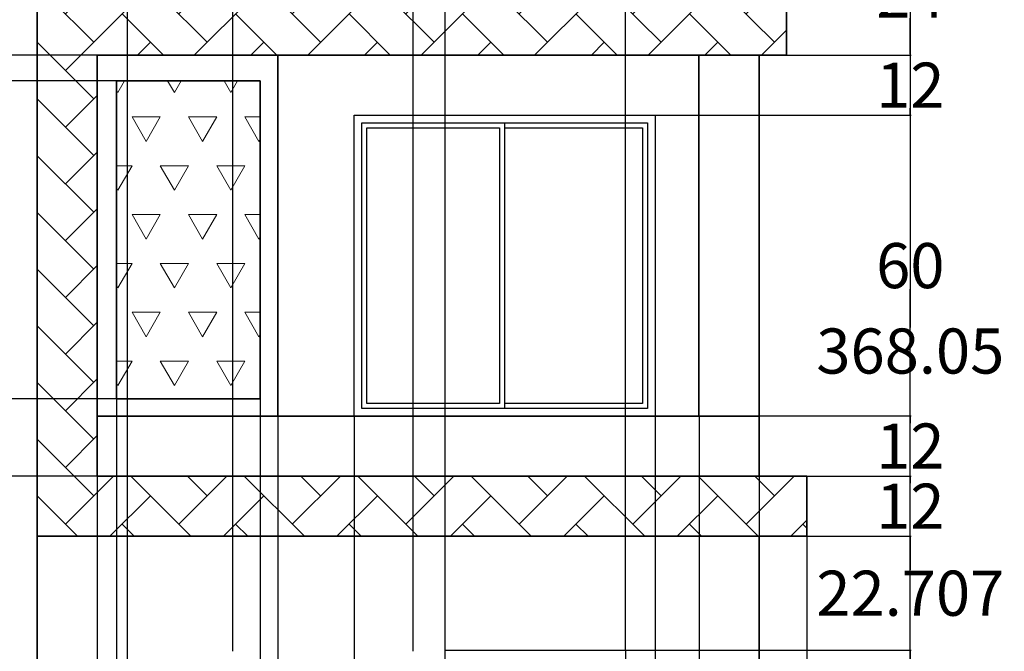
# Model space of a CAD drawing. Units: inches. Extents: x -30 to 323, y -174 to 256.
# Tile 3 of 4: x 127 to 323, y -14 to 112. Entities that reach past the tile are written whole.
import ezdxf

# ---------------------------------------------------------------- set-up
doc = ezdxf.new("R2010")
doc.units = ezdxf.units.IN
doc.header["$MEASUREMENT"] = 0
for name, color, linetype, lineweight in [('A-ANNO-DIMS', 2, 'Continuous', 18), ('A-ELEV', 7, 'Continuous', 35), ('A-ELEV-PATT', 8, 'Continuous', 13), ('A-GLAZ', 3, 'Continuous', 25)]:
    doc.layers.add(name, color=color, linetype=linetype, lineweight=lineweight)
doc.styles.get("Standard").update_dxf_attribs({"font": 'arial.ttf'})
doc.dimstyles.get("Standard").update_dxf_attribs({"dimtxt": 9, "dimasz": 0.18, "dimexe": 0.18, "dimexo": 0.0625, "dimgap": 0.09, "dimtad": 0, "dimtih": 1, "dimtoh": 1, "dimdec": 0, "dimzin": 0, "dimdsep": 46, "dimlunit": 3, "dimtxsty": 'Standard', "dimcen": 0.09, "dimadec": 0, "dimazin": 0, "dimtfac": 1, "dimtdec": 0, "dimtofl": 0, "dimtmove": 0, "dimatfit": 3, "dimfxl": 1, "dimtolj": 1, "dimtzin": 0, "dimarcsym": 0})

# ---------------------------------------------------------------- blocks, each defined once
blk = doc.blocks.new('*U5')
for p, q in [((1.5, 1.5), (1.5, 58.5)), ((1.5, 58.5), (30, 58.5)), ((30, 1.5), (30, 58.5)), ((30, 58.5), (58.5, 58.5)), ((58.5, 58.5), (58.5, 1.5)), ((30, 1.5), (1.5, 1.5)), ((58.5, 1.5), (30, 1.5))]:
    blk.add_line(p, q)
blk.add_lwpolyline([(0, 0), (0, 60), (60, 60), (60, 0)], close=True)
for points in [[(29, 57.5), (29, 2.5), (2.5, 2.5), (2.5, 57.5), (29, 57.5)], [(30, 57.5), (57.5, 57.5), (57.5, 2.5), (30, 2.5)]]:
    blk.add_lwpolyline(points)
blk = doc.blocks.new('*D9')
at = {"layer": 'A-ANNO-DIMS', "color": 0, "lineweight": -2, "transparency": 16777216}
for p, q in [((283.63, 8.84), (283.63, -158.98)), ((22.14, -138.22), (22.14, -158.98)), ((22.32, -158.8), (137.5, -158.8)), ((283.45, -158.8), (168.27, -158.8))]:
    blk.add_line(p, q, dxfattribs=at)
at = {"layer": 'A-ANNO-DIMS', "color": 0, "transparency": 16777216}
for points in [[(22.32, -158.77), (22.32, -158.83), (22.14, -158.8)], [(283.45, -158.77), (283.45, -158.83), (283.63, -158.8)]]:
    blk.add_solid(points, dxfattribs=at)
at = {"layer": 'Defpoints', "color": 0, "transparency": 16777216}
for p in [(283.63, 8.91), (22.14, -138.15), (283.63, -158.8)]:
    blk.add_point(p, dxfattribs=at)
at = {"layer": 'A-ANNO-DIMS', "color": 0, "transparency": 16777216, "insert": (152.88, -158.8), "char_height": 9, "attachment_point": 5}
blk.add_mtext('\\A1;261.5', dxfattribs=at)
blk = doc.blocks.new('*D10')
at = {"layer": 'A-ANNO-DIMS', "color": 0, "lineweight": -2, "transparency": 16777216}
for p, q in [((15.03, 229.9), (304.46, 229.9)), ((304.28, 229.72), (304.28, 50.56)), ((304.28, -137.97), (304.28, 41.18)), ((22.2, -138.15), (304.46, -138.15))]:
    blk.add_line(p, q, dxfattribs=at)
at = {"layer": 'A-ANNO-DIMS', "color": 0, "transparency": 16777216}
for points in [[(304.25, 229.72), (304.31, 229.72), (304.28, 229.9)], [(304.25, -137.97), (304.31, -137.97), (304.28, -138.15)]]:
    blk.add_solid(points, dxfattribs=at)
at = {"layer": 'Defpoints', "color": 0, "transparency": 16777216}
for p in [(14.97, 229.9), (22.14, -138.15), (304.28, -138.15)]:
    blk.add_point(p, dxfattribs=at)
at = {"layer": 'A-ANNO-DIMS', "color": 0, "transparency": 16777216, "insert": (304.28, 45.87), "char_height": 9, "attachment_point": 5}
blk.add_mtext('\\A1;368.05', dxfattribs=at)
blk = doc.blocks.new('*D22')
at = {"layer": 'A-ANNO-DIMS', "color": 0, "lineweight": -2, "transparency": 16777216}
for p, q in [((92.12, -60.62), (92.12, 250.73)), ((92.3, 250.55), (95.9, 250.55)), ((129.96, 250.55), (126.35, 250.55)), ((130.14, -111.03), (130.14, 250.73))]:
    blk.add_line(p, q, dxfattribs=at)
at = {"layer": 'A-ANNO-DIMS', "color": 0, "transparency": 16777216}
for points in [[(92.3, 250.58), (92.3, 250.52), (92.12, 250.55)], [(129.96, 250.58), (129.96, 250.52), (130.14, 250.55)]]:
    blk.add_solid(points, dxfattribs=at)
at = {"layer": 'Defpoints', "color": 0, "transparency": 16777216}
for p in [(130.14, 250.55), (92.12, -60.68), (130.14, -111.09)]:
    blk.add_point(p, dxfattribs=at)
at = {"layer": 'A-ANNO-DIMS', "color": 0, "transparency": 16777216, "insert": (111.13, 250.55), "char_height": 9, "attachment_point": 5}
blk.add_mtext('\\A1;38.02', dxfattribs=at)
blk = doc.blocks.new('*D44')
at = {"layer": 'A-ANNO-DIMS', "color": 0, "lineweight": -2, "transparency": 16777216}
for p, q in [((142.14, 20.84), (142.14, -158.98)), ((130.14, 8.84), (130.14, -158.98)), ((130.32, -158.8), (141.96, -158.8)), ((142.14, -158.8), (142.32, -158.8))]:
    blk.add_line(p, q, dxfattribs=at)
at = {"layer": 'A-ANNO-DIMS', "color": 0, "transparency": 16777216}
for points in [[(130.32, -158.77), (130.32, -158.83), (130.14, -158.8)], [(141.96, -158.77), (141.96, -158.83), (142.14, -158.8)]]:
    blk.add_solid(points, dxfattribs=at)
at = {"layer": 'Defpoints', "color": 0, "transparency": 16777216}
for p in [(142.14, 20.91), (130.14, 8.91), (142.14, -158.8)]:
    blk.add_point(p, dxfattribs=at)
at = {"layer": 'A-ANNO-DIMS', "color": 0, "transparency": 16777216, "insert": (148.38, -158.8), "char_height": 9, "attachment_point": 5}
blk.add_mtext('\\A1;12', dxfattribs=at)
blk = doc.blocks.new('*D45')
at = {"layer": 'A-ANNO-DIMS', "color": 0, "lineweight": -2, "transparency": 16777216}
for p, q in [((145.99, 36.26), (145.99, -158.98)), ((142.14, 20.84), (142.14, -158.98)), ((142.32, -158.8), (145.81, -158.8)), ((145.99, -158.8), (146.17, -158.8))]:
    blk.add_line(p, q, dxfattribs=at)
at = {"layer": 'A-ANNO-DIMS', "color": 0, "transparency": 16777216}
for points in [[(142.32, -158.77), (142.32, -158.83), (142.14, -158.8)], [(145.81, -158.77), (145.81, -158.83), (145.99, -158.8)]]:
    blk.add_solid(points, dxfattribs=at)
at = {"layer": 'Defpoints', "color": 0, "transparency": 16777216}
for p in [(145.99, 36.33), (142.14, 20.91), (145.99, -158.8)]:
    blk.add_point(p, dxfattribs=at)
at = {"layer": 'A-ANNO-DIMS', "color": 0, "transparency": 16777216, "insert": (157.98, -158.8), "char_height": 9, "attachment_point": 5}
blk.add_mtext('\\A1;3.85', dxfattribs=at)
blk = doc.blocks.new('*D46')
at = {"layer": 'A-ANNO-DIMS', "color": 0, "lineweight": -2, "transparency": 16777216}
for p, q in [((145.99, 36.26), (145.99, -158.98)), ((174.62, 36.26), (174.62, -158.98)), ((146.17, -158.8), (174.44, -158.8)), ((174.62, -158.8), (174.8, -158.8))]:
    blk.add_line(p, q, dxfattribs=at)
at = {"layer": 'A-ANNO-DIMS', "color": 0, "transparency": 16777216}
for points in [[(146.17, -158.77), (146.17, -158.83), (145.99, -158.8)], [(174.44, -158.77), (174.44, -158.83), (174.62, -158.8)]]:
    blk.add_solid(points, dxfattribs=at)
at = {"layer": 'Defpoints', "color": 0, "transparency": 16777216}
for p in [(145.99, 36.33), (174.62, 36.33), (174.62, -158.8)]:
    blk.add_point(p, dxfattribs=at)
at = {"layer": 'A-ANNO-DIMS', "color": 0, "transparency": 16777216, "insert": (190.15, -158.8), "char_height": 9, "attachment_point": 5}
blk.add_mtext('\\A1;28.63', dxfattribs=at)
blk = doc.blocks.new('*D47')
at = {"layer": 'A-ANNO-DIMS', "color": 0, "lineweight": -2, "transparency": 16777216}
for p, q in [((174.62, 36.26), (174.62, -158.98)), ((178.14, 32.84), (178.14, -158.98)), ((174.8, -158.8), (177.96, -158.8)), ((178.14, -158.8), (178.32, -158.8))]:
    blk.add_line(p, q, dxfattribs=at)
at = {"layer": 'A-ANNO-DIMS', "color": 0, "transparency": 16777216}
for points in [[(174.8, -158.77), (174.8, -158.83), (174.62, -158.8)], [(177.96, -158.77), (177.96, -158.83), (178.14, -158.8)]]:
    blk.add_solid(points, dxfattribs=at)
at = {"layer": 'Defpoints', "color": 0, "transparency": 16777216}
for p in [(174.62, 36.33), (178.14, 32.91), (178.14, -158.8)]:
    blk.add_point(p, dxfattribs=at)
at = {"layer": 'A-ANNO-DIMS', "color": 0, "transparency": 16777216, "insert": (193.6, -158.8), "char_height": 9, "attachment_point": 5}
blk.add_mtext('\\A1;3.518', dxfattribs=at)
blk = doc.blocks.new('*D48')
at = {"layer": 'A-ANNO-DIMS', "color": 0, "lineweight": -2, "transparency": 16777216}
for p, q in [((178.14, 32.84), (178.14, -158.98)), ((193.38, 32.84), (193.38, -158.98)), ((178.32, -158.8), (193.2, -158.8)), ((193.38, -158.8), (193.56, -158.8))]:
    blk.add_line(p, q, dxfattribs=at)
at = {"layer": 'A-ANNO-DIMS', "color": 0, "transparency": 16777216}
for points in [[(178.32, -158.77), (178.32, -158.83), (178.14, -158.8)], [(193.2, -158.77), (193.2, -158.83), (193.38, -158.8)]]:
    blk.add_solid(points, dxfattribs=at)
at = {"layer": 'Defpoints', "color": 0, "transparency": 16777216}
for p in [(178.14, 32.91), (193.38, 32.91), (193.38, -158.8)]:
    blk.add_point(p, dxfattribs=at)
at = {"layer": 'A-ANNO-DIMS', "color": 0, "transparency": 16777216, "insert": (211.91, -158.8), "char_height": 9, "attachment_point": 5}
blk.add_mtext('\\A1;15.247', dxfattribs=at)
blk = doc.blocks.new('*D49')
at = {"layer": 'A-ANNO-DIMS', "color": 0, "lineweight": -2, "transparency": 16777216}
for p, q in [((193.38, 32.84), (193.38, -158.98)), ((253.38, 32.84), (253.38, -158.98)), ((193.56, -158.8), (216.84, -158.8)), ((253.2, -158.8), (229.93, -158.8))]:
    blk.add_line(p, q, dxfattribs=at)
at = {"layer": 'A-ANNO-DIMS', "color": 0, "transparency": 16777216}
for points in [[(193.56, -158.77), (193.56, -158.83), (193.38, -158.8)], [(253.2, -158.77), (253.2, -158.83), (253.38, -158.8)]]:
    blk.add_solid(points, dxfattribs=at)
at = {"layer": 'Defpoints', "color": 0, "transparency": 16777216}
for p in [(193.38, 32.91), (253.38, 32.91), (253.38, -158.8)]:
    blk.add_point(p, dxfattribs=at)
at = {"layer": 'A-ANNO-DIMS', "color": 0, "transparency": 16777216, "insert": (223.38, -158.8), "char_height": 9, "attachment_point": 5}
blk.add_mtext('\\A1;60', dxfattribs=at)
blk = doc.blocks.new('*D50')
at = {"layer": 'A-ANNO-DIMS', "color": 0, "lineweight": -2, "transparency": 16777216}
for p, q in [((253.38, 32.84), (253.38, -158.98)), ((262.14, 32.84), (262.14, -158.98)), ((253.56, -158.8), (261.96, -158.8)), ((262.14, -158.8), (262.32, -158.8))]:
    blk.add_line(p, q, dxfattribs=at)
at = {"layer": 'A-ANNO-DIMS', "color": 0, "transparency": 16777216}
for points in [[(253.56, -158.77), (253.56, -158.83), (253.38, -158.8)], [(261.96, -158.77), (261.96, -158.83), (262.14, -158.8)]]:
    blk.add_solid(points, dxfattribs=at)
at = {"layer": 'Defpoints', "color": 0, "transparency": 16777216}
for p in [(253.38, 32.91), (262.14, 32.91), (262.14, -158.8)]:
    blk.add_point(p, dxfattribs=at)
at = {"layer": 'A-ANNO-DIMS', "color": 0, "transparency": 16777216, "insert": (277.6, -158.8), "char_height": 9, "attachment_point": 5}
blk.add_mtext('\\A1;8.753', dxfattribs=at)
blk = doc.blocks.new('*D51')
at = {"layer": 'A-ANNO-DIMS', "color": 0, "lineweight": -2, "transparency": 16777216}
for p, q in [((262.14, 32.84), (262.14, -158.98)), ((274.14, 20.84), (274.14, -158.98)), ((262.32, -158.8), (273.96, -158.8)), ((274.14, -158.8), (274.32, -158.8))]:
    blk.add_line(p, q, dxfattribs=at)
at = {"layer": 'A-ANNO-DIMS', "color": 0, "transparency": 16777216}
for points in [[(262.32, -158.77), (262.32, -158.83), (262.14, -158.8)], [(273.96, -158.77), (273.96, -158.83), (274.14, -158.8)]]:
    blk.add_solid(points, dxfattribs=at)
at = {"layer": 'Defpoints', "color": 0, "transparency": 16777216}
for p in [(262.14, 32.91), (274.14, 20.91), (274.14, -158.8)]:
    blk.add_point(p, dxfattribs=at)
at = {"layer": 'A-ANNO-DIMS', "color": 0, "transparency": 16777216, "insert": (280.38, -158.8), "char_height": 9, "attachment_point": 5}
blk.add_mtext('\\A1;12', dxfattribs=at)
blk = doc.blocks.new('*D52')
at = {"layer": 'A-ANNO-DIMS', "color": 0, "lineweight": -2, "transparency": 16777216}
for p, q in [((148.14, -47.95), (148.14, 250.73)), ((148.32, 250.55), (168.97, 250.55)), ((169.15, -13.98), (169.15, 250.73)), ((169.15, 250.55), (169.33, 250.55))]:
    blk.add_line(p, q, dxfattribs=at)
at = {"layer": 'A-ANNO-DIMS', "color": 0, "transparency": 16777216}
for points in [[(148.32, 250.58), (148.32, 250.52), (148.14, 250.55)], [(168.97, 250.58), (168.97, 250.52), (169.15, 250.55)]]:
    blk.add_solid(points, dxfattribs=at)
at = {"layer": 'Defpoints', "color": 0, "transparency": 16777216}
for p in [(169.15, 250.55), (169.15, -14.04), (148.14, -48.01)]:
    blk.add_point(p, dxfattribs=at)
at = {"layer": 'A-ANNO-DIMS', "color": 0, "transparency": 16777216, "insert": (188.16, 250.55), "char_height": 9, "attachment_point": 5}
blk.add_mtext('\\A1;21.014', dxfattribs=at)
blk = doc.blocks.new('*D53')
at = {"layer": 'A-ANNO-DIMS', "color": 0, "lineweight": -2, "transparency": 16777216}
for p, q in [((169.15, -13.98), (169.15, 250.73)), ((169.33, 250.55), (180.62, 250.55)), ((204.97, 250.55), (193.68, 250.55)), ((205.15, -13.98), (205.15, 250.73))]:
    blk.add_line(p, q, dxfattribs=at)
at = {"layer": 'A-ANNO-DIMS', "color": 0, "transparency": 16777216}
for points in [[(169.33, 250.58), (169.33, 250.52), (169.15, 250.55)], [(204.97, 250.58), (204.97, 250.52), (205.15, 250.55)]]:
    blk.add_solid(points, dxfattribs=at)
at = {"layer": 'Defpoints', "color": 0, "transparency": 16777216}
for p in [(205.15, 250.55), (169.15, -14.04), (205.15, -14.04)]:
    blk.add_point(p, dxfattribs=at)
at = {"layer": 'A-ANNO-DIMS', "color": 0, "transparency": 16777216, "insert": (187.15, 250.55), "char_height": 9, "attachment_point": 5}
blk.add_mtext('\\A1;36', dxfattribs=at)
blk = doc.blocks.new('*D54')
at = {"layer": 'A-ANNO-DIMS', "color": 0, "lineweight": -2, "transparency": 16777216}
for p, q in [((205.15, -13.98), (205.15, 250.73)), ((205.33, 250.55), (211.31, 250.55)), ((211.49, -13.74), (211.49, 250.73)), ((211.49, 250.55), (211.67, 250.55))]:
    blk.add_line(p, q, dxfattribs=at)
at = {"layer": 'A-ANNO-DIMS', "color": 0, "transparency": 16777216}
for points in [[(205.33, 250.58), (205.33, 250.52), (205.15, 250.55)], [(211.31, 250.58), (211.31, 250.52), (211.49, 250.55)]]:
    blk.add_solid(points, dxfattribs=at)
at = {"layer": 'Defpoints', "color": 0, "transparency": 16777216}
for p in [(211.49, 250.55), (205.15, -14.04), (211.49, -13.8)]:
    blk.add_point(p, dxfattribs=at)
at = {"layer": 'A-ANNO-DIMS', "color": 0, "transparency": 16777216, "insert": (226.98, 250.55), "char_height": 9, "attachment_point": 5}
blk.add_mtext('\\A1;6.338', dxfattribs=at)
blk = doc.blocks.new('*D55')
at = {"layer": 'A-ANNO-DIMS', "color": 0, "lineweight": -2, "transparency": 16777216}
for p, q in [((211.49, -13.74), (211.49, 250.73)), ((211.67, 250.55), (222.96, 250.55)), ((247.31, 250.55), (236.02, 250.55)), ((247.49, -13.74), (247.49, 250.73))]:
    blk.add_line(p, q, dxfattribs=at)
at = {"layer": 'A-ANNO-DIMS', "color": 0, "transparency": 16777216}
for points in [[(211.67, 250.58), (211.67, 250.52), (211.49, 250.55)], [(247.31, 250.58), (247.31, 250.52), (247.49, 250.55)]]:
    blk.add_solid(points, dxfattribs=at)
at = {"layer": 'Defpoints', "color": 0, "transparency": 16777216}
for p in [(247.49, 250.55), (211.49, -13.8), (247.49, -13.8)]:
    blk.add_point(p, dxfattribs=at)
at = {"layer": 'A-ANNO-DIMS', "color": 0, "transparency": 16777216, "insert": (229.49, 250.55), "char_height": 9, "attachment_point": 5}
blk.add_mtext('\\A1;36', dxfattribs=at)
blk = doc.blocks.new('*D60')
at = {"layer": 'A-ANNO-DIMS', "color": 0, "lineweight": -2, "transparency": 16777216}
for p, q in [((283.63, 8.84), (283.63, -158.98)), ((274.14, -111.16), (274.14, -158.98)), ((274.32, -158.8), (283.45, -158.8)), ((283.63, -158.8), (283.81, -158.8))]:
    blk.add_line(p, q, dxfattribs=at)
at = {"layer": 'A-ANNO-DIMS', "color": 0, "transparency": 16777216}
for points in [[(274.32, -158.77), (274.32, -158.83), (274.14, -158.8)], [(283.45, -158.77), (283.45, -158.83), (283.63, -158.8)]]:
    blk.add_solid(points, dxfattribs=at)
at = {"layer": 'Defpoints', "color": 0, "transparency": 16777216}
for p in [(283.63, 8.91), (274.14, -111.09), (283.63, -158.8)]:
    blk.add_point(p, dxfattribs=at)
at = {"layer": 'A-ANNO-DIMS', "color": 0, "transparency": 16777216, "insert": (299.09, -158.8), "char_height": 9, "attachment_point": 5}
blk.add_mtext('\\A1;9.497', dxfattribs=at)
blk = doc.blocks.new('*D63')
at = {"layer": 'A-ANNO-DIMS', "color": 0, "lineweight": -2, "transparency": 16777216}
for p, q in [((247.55, -13.8), (304.46, -13.8)), ((304.28, -13.98), (304.28, -26.22)), ((304.28, -47.83), (304.28, -35.59)), ((256.2, -48.01), (304.46, -48.01))]:
    blk.add_line(p, q, dxfattribs=at)
at = {"layer": 'A-ANNO-DIMS', "color": 0, "transparency": 16777216}
for points in [[(304.25, -13.98), (304.31, -13.98), (304.28, -13.8)], [(304.25, -47.83), (304.31, -47.83), (304.28, -48.01)]]:
    blk.add_solid(points, dxfattribs=at)
at = {"layer": 'Defpoints', "color": 0, "transparency": 16777216}
for p in [(247.49, -13.8), (304.28, -13.8), (256.14, -48.01)]:
    blk.add_point(p, dxfattribs=at)
at = {"layer": 'A-ANNO-DIMS', "color": 0, "transparency": 16777216, "insert": (304.28, -30.9), "char_height": 9, "attachment_point": 5}
blk.add_mtext('\\A1;34.21', dxfattribs=at)
blk = doc.blocks.new('*D64')
at = {"layer": 'A-ANNO-DIMS', "color": 0, "lineweight": -2, "transparency": 16777216}
for p, q in [((283.7, 8.91), (304.46, 8.91)), ((304.28, 8.73), (304.28, 2.24)), ((304.28, -13.62), (304.28, -7.13)), ((247.55, -13.8), (304.46, -13.8))]:
    blk.add_line(p, q, dxfattribs=at)
at = {"layer": 'A-ANNO-DIMS', "color": 0, "transparency": 16777216}
for points in [[(304.25, 8.73), (304.31, 8.73), (304.28, 8.91)], [(304.25, -13.62), (304.31, -13.62), (304.28, -13.8)]]:
    blk.add_solid(points, dxfattribs=at)
at = {"layer": 'Defpoints', "color": 0, "transparency": 16777216}
for p in [(283.63, 8.91), (304.28, 8.91), (247.49, -13.8)]:
    blk.add_point(p, dxfattribs=at)
at = {"layer": 'A-ANNO-DIMS', "color": 0, "transparency": 16777216, "insert": (304.28, -2.45), "char_height": 9, "attachment_point": 5}
blk.add_mtext('\\A1;22.707', dxfattribs=at)
blk = doc.blocks.new('*D65')
at = {"layer": 'A-ANNO-DIMS', "color": 0, "lineweight": -2, "transparency": 16777216}
for p, q in [((283.7, 20.91), (304.46, 20.91)), ((304.28, 20.73), (304.28, 19.51)), ((304.28, 9.09), (304.28, 10.3)), ((283.7, 8.91), (304.46, 8.91))]:
    blk.add_line(p, q, dxfattribs=at)
at = {"layer": 'A-ANNO-DIMS', "color": 0, "transparency": 16777216}
for points in [[(304.25, 20.73), (304.31, 20.73), (304.28, 20.91)], [(304.25, 9.09), (304.31, 9.09), (304.28, 8.91)]]:
    blk.add_solid(points, dxfattribs=at)
at = {"layer": 'Defpoints', "color": 0, "transparency": 16777216}
for p in [(283.63, 20.91), (304.28, 20.91), (283.63, 8.91)]:
    blk.add_point(p, dxfattribs=at)
at = {"layer": 'A-ANNO-DIMS', "color": 0, "transparency": 16777216, "insert": (304.28, 14.91), "char_height": 9, "attachment_point": 5}
blk.add_mtext('\\A1;12', dxfattribs=at)
blk = doc.blocks.new('*D66')
at = {"layer": 'A-ANNO-DIMS', "color": 0, "lineweight": -2, "transparency": 16777216}
for p, q in [((274.2, 32.91), (304.46, 32.91)), ((304.28, 32.73), (304.28, 31.51)), ((304.28, 21.09), (304.28, 22.3)), ((274.2, 20.91), (304.46, 20.91))]:
    blk.add_line(p, q, dxfattribs=at)
at = {"layer": 'A-ANNO-DIMS', "color": 0, "transparency": 16777216}
for points in [[(304.25, 32.73), (304.31, 32.73), (304.28, 32.91)], [(304.25, 21.09), (304.31, 21.09), (304.28, 20.91)]]:
    blk.add_solid(points, dxfattribs=at)
at = {"layer": 'Defpoints', "color": 0, "transparency": 16777216}
for p in [(274.14, 32.91), (304.28, 32.91), (274.14, 20.91)]:
    blk.add_point(p, dxfattribs=at)
at = {"layer": 'A-ANNO-DIMS', "color": 0, "transparency": 16777216, "insert": (304.28, 26.91), "char_height": 9, "attachment_point": 5}
blk.add_mtext('\\A1;12', dxfattribs=at)
blk = doc.blocks.new('*D67')
at = {"layer": 'A-ANNO-DIMS', "color": 0, "lineweight": -2, "transparency": 16777216}
for p, q in [((253.45, 92.91), (304.46, 92.91)), ((304.28, 92.73), (304.28, 67.59)), ((304.28, 33.09), (304.28, 58.22)), ((274.2, 32.91), (304.46, 32.91))]:
    blk.add_line(p, q, dxfattribs=at)
at = {"layer": 'A-ANNO-DIMS', "color": 0, "transparency": 16777216}
for points in [[(304.25, 92.73), (304.31, 92.73), (304.28, 92.91)], [(304.25, 33.09), (304.31, 33.09), (304.28, 32.91)]]:
    blk.add_solid(points, dxfattribs=at)
at = {"layer": 'Defpoints', "color": 0, "transparency": 16777216}
for p in [(253.38, 92.91), (304.28, 92.91), (274.14, 32.91)]:
    blk.add_point(p, dxfattribs=at)
at = {"layer": 'A-ANNO-DIMS', "color": 0, "transparency": 16777216, "insert": (304.28, 62.91), "char_height": 9, "attachment_point": 5}
blk.add_mtext('\\A1;60', dxfattribs=at)
blk = doc.blocks.new('*D68')
at = {"layer": 'A-ANNO-DIMS', "color": 0, "lineweight": -2, "transparency": 16777216}
for p, q in [((274.2, 104.91), (304.46, 104.91)), ((304.28, 104.73), (304.28, 103.51)), ((304.28, 93.09), (304.28, 94.3)), ((253.45, 92.91), (304.46, 92.91))]:
    blk.add_line(p, q, dxfattribs=at)
at = {"layer": 'A-ANNO-DIMS', "color": 0, "transparency": 16777216}
for points in [[(304.25, 104.73), (304.31, 104.73), (304.28, 104.91)], [(304.25, 93.09), (304.31, 93.09), (304.28, 92.91)]]:
    blk.add_solid(points, dxfattribs=at)
at = {"layer": 'Defpoints', "color": 0, "transparency": 16777216}
for p in [(274.14, 104.91), (304.28, 104.91), (253.38, 92.91)]:
    blk.add_point(p, dxfattribs=at)
at = {"layer": 'A-ANNO-DIMS', "color": 0, "transparency": 16777216, "insert": (304.28, 98.91), "char_height": 9, "attachment_point": 5}
blk.add_mtext('\\A1;12', dxfattribs=at)
blk = doc.blocks.new('*D69')
at = {"layer": 'A-ANNO-DIMS', "color": 0, "lineweight": -2, "transparency": 16777216}
for p, q in [((279.63, 128.91), (304.46, 128.91)), ((304.28, 128.73), (304.28, 121.51)), ((304.28, 105.09), (304.28, 112.3)), ((279.63, 104.91), (304.46, 104.91))]:
    blk.add_line(p, q, dxfattribs=at)
at = {"layer": 'A-ANNO-DIMS', "color": 0, "transparency": 16777216}
for points in [[(304.25, 128.73), (304.31, 128.73), (304.28, 128.91)], [(304.25, 105.09), (304.31, 105.09), (304.28, 104.91)]]:
    blk.add_solid(points, dxfattribs=at)
at = {"layer": 'Defpoints', "color": 0, "transparency": 16777216}
for p in [(279.57, 128.91), (304.28, 128.91), (279.57, 104.91)]:
    blk.add_point(p, dxfattribs=at)
at = {"layer": 'A-ANNO-DIMS', "color": 0, "transparency": 16777216, "insert": (304.28, 116.91), "char_height": 9, "attachment_point": 5}
blk.add_mtext('\\A1;24', dxfattribs=at)
blk = doc.blocks.new('*D74')
at = {"layer": 'A-ANNO-DIMS', "color": 0, "lineweight": -2, "transparency": 16777216}
for p, q in [((145.92, 36.33), (-5.86, 36.33)), ((-5.68, 36.15), (-5.68, 33.3)), ((-5.68, 21.09), (-5.68, 23.93)), ((142.07, 20.91), (-5.86, 20.91))]:
    blk.add_line(p, q, dxfattribs=at)
at = {"layer": 'A-ANNO-DIMS', "color": 0, "transparency": 16777216}
for points in [[(-5.71, 36.15), (-5.65, 36.15), (-5.68, 36.33)], [(-5.71, 21.09), (-5.65, 21.09), (-5.68, 20.91)]]:
    blk.add_solid(points, dxfattribs=at)
at = {"layer": 'Defpoints', "color": 0, "transparency": 16777216}
for p in [(-5.68, 36.33), (145.99, 36.33), (142.14, 20.91)]:
    blk.add_point(p, dxfattribs=at)
at = {"layer": 'A-ANNO-DIMS', "color": 0, "transparency": 16777216, "insert": (-5.68, 28.62), "char_height": 9, "attachment_point": 5}
blk.add_mtext('\\A1;15.42', dxfattribs=at)
blk = doc.blocks.new('*D75')
at = {"layer": 'A-ANNO-DIMS', "color": 0, "lineweight": -2, "transparency": 16777216}
for p, q in [((145.92, 99.75), (-5.86, 99.75)), ((-5.68, 99.57), (-5.68, 72.73)), ((-5.68, 36.51), (-5.68, 63.35)), ((145.92, 36.33), (-5.86, 36.33))]:
    blk.add_line(p, q, dxfattribs=at)
at = {"layer": 'A-ANNO-DIMS', "color": 0, "transparency": 16777216}
for points in [[(-5.71, 99.57), (-5.65, 99.57), (-5.68, 99.75)], [(-5.71, 36.51), (-5.65, 36.51), (-5.68, 36.33)]]:
    blk.add_solid(points, dxfattribs=at)
at = {"layer": 'Defpoints', "color": 0, "transparency": 16777216}
for p in [(-5.68, 99.75), (145.99, 99.75), (145.99, 36.33)]:
    blk.add_point(p, dxfattribs=at)
at = {"layer": 'A-ANNO-DIMS', "color": 0, "transparency": 16777216, "insert": (-5.68, 68.04), "char_height": 9, "attachment_point": 5}
blk.add_mtext('\\A1;63.43', dxfattribs=at)
blk = doc.blocks.new('*D76')
at = {"layer": 'A-ANNO-DIMS', "color": 0, "lineweight": -2, "transparency": 16777216}
for p, q in [((142.07, 104.91), (-5.86, 104.91)), ((-5.68, 104.91), (-5.68, 105.09)), ((-5.68, 105.09), (-5.5, 105.09)), ((-5.68, 99.93), (-5.68, 104.73)), ((145.92, 99.75), (-5.86, 99.75))]:
    blk.add_line(p, q, dxfattribs=at)
at = {"layer": 'A-ANNO-DIMS', "color": 0, "transparency": 16777216}
for points in [[(-5.71, 104.73), (-5.65, 104.73), (-5.68, 104.91)], [(-5.71, 99.93), (-5.65, 99.93), (-5.68, 99.75)]]:
    blk.add_solid(points, dxfattribs=at)
at = {"layer": 'Defpoints', "color": 0, "transparency": 16777216}
for p in [(-5.68, 104.91), (142.14, 104.91), (145.99, 99.75)]:
    blk.add_point(p, dxfattribs=at)
at = {"layer": 'A-ANNO-DIMS', "color": 0, "transparency": 16777216, "insert": (9.73, 105.09), "char_height": 9, "attachment_point": 5}
blk.add_mtext('\\A1;5.152', dxfattribs=at)

msp = doc.modelspace()

# ---------------------------------------------------------------- hatches: boundary and pattern name
at = {"layer": 'A-ELEV-PATT'}
h = msp.add_hatch(dxfattribs=at)
h.set_pattern_fill('AR-HBONE', color=256, scale=2)
h.paths.add_polyline_path([(279.5695, 128.9059), (274.136, 128.9059), (130.136, 128.9059), (130.136, 8.9059), (274.136, 8.9059), (283.6325, 8.9059), (283.6325, 20.9059), (274.136, 20.9059), (142.136, 20.9059), (142.136, 104.9059), (274.136, 104.9059), (279.5695, 104.9059)])
h = msp.add_hatch(dxfattribs=at)
h.set_pattern_fill('TRIANG', color=256, scale=30)
h.paths.add_polyline_path([(174.6182, 99.7543), (145.9862, 99.7543), (145.9862, 36.3257), (174.6182, 36.3257)])

# ---------------------------------------------------------------- linework, layer by layer
at = {"layer": 'A-ELEV'}
for p, q in [((178.136, 104.9059), (178.136, 32.9059)), ((262.136, 32.9059), (262.136, 104.9059)), ((142.136, 32.9059), (274.136, 32.9059)), ((130.136, 8.9059), (274.136, 8.9059))]:
    msp.add_line(p, q, dxfattribs=at)
for points in [[(130.136, 149.9059), (274.136, 149.9059), (274.136, 128.9059), (279.5695, 128.9059), (279.5695, 104.9059), (274.136, 104.9059), (274.136, 20.9059), (283.6325, 20.9059), (283.6325, 8.9059), (274.136, 8.9059), (274.136, -111.0941), (22.136, -111.0941), (22.136, 224.9059), (130.136, 224.9059), (130.136, -111.0941)], [(274.136, 104.9059), (142.136, 104.9059), (142.136, 20.9059), (274.136, 20.9059)]]:
    msp.add_lwpolyline(points, dxfattribs=at)
msp.add_lwpolyline([(145.9862, 99.7543), (174.6182, 99.7543), (174.6182, 36.3257), (145.9862, 36.3257)], close=True, dxfattribs=at)
at = {"layer": 'A-GLAZ'}
msp.add_lwpolyline([(211.4887, -48.0084), (211.4887, -13.801), (247.4887, -13.801), (247.4887, -48.0084)], dxfattribs=at)

# ---------------------------------------------------------------- block references
msp.add_blockref('*U5', (193.3831, 32.9059), dxfattribs=at)

# ---------------------------------------------------------------- dimensions: what is measured, and where the dimension line sits
at = {"layer": 'A-ANNO-DIMS'}
for base, p1, p2, override, picture, middle in [((130.136, 250.5457), (92.1189, -60.6838), (130.136, -111.0941), {"dimdec": 2, "dimlfac": 1, "dimrnd": 0, "dimzin": 0, "dimdsep": 46, "dimlunit": 2}, '*D22', (111.1274, 250.5457)), ((169.1503, 250.5457), (148.136, -48.0084), (169.1503, -14.04), {"dimdec": 3, "dimlfac": 1, "dimrnd": 0, "dimzin": 0, "dimdsep": 46, "dimlunit": 2}, '*D52', (188.1601, 250.5457)), ((205.1503, 250.5457), (169.1503, -14.04), (205.1503, -14.04), {"dimdec": 0, "dimlfac": 1, "dimrnd": 0, "dimzin": 0, "dimdsep": 46, "dimlunit": 2}, '*D53', (187.1503, 250.5457)), ((211.4887, 250.5457), (205.1503, -14.04), (211.4887, -13.801), {"dimdec": 3, "dimlfac": 1, "dimrnd": 0, "dimzin": 0, "dimdsep": 46, "dimlunit": 2}, '*D54', (226.9777, 250.5457)), ((247.4887, 250.5457), (211.4887, -13.801), (247.4887, -13.801), {"dimdec": 0, "dimlfac": 1, "dimrnd": 0, "dimzin": 0, "dimdsep": 46, "dimlunit": 2}, '*D55', (229.4887, 250.5457)), ((145.9862, -158.8026), (142.136, 20.9059), (145.9862, 36.3257), {"dimdec": 2, "dimlfac": 1, "dimrnd": 0, "dimzin": 0, "dimdsep": 46, "dimlunit": 2}, '*D45', (157.9758, -158.8026)), ((174.6182, -158.8026), (145.9862, 36.3257), (174.6182, 36.3257), {"dimdec": 2, "dimlfac": 1, "dimrnd": 0, "dimzin": 0, "dimdsep": 46, "dimlunit": 2}, '*D46', (190.1501, -158.8026)), ((178.136, -158.8026), (174.6182, 36.3257), (178.136, 32.9059), {"dimdec": 3, "dimlfac": 1, "dimrnd": 0, "dimzin": 0, "dimdsep": 46, "dimlunit": 2}, '*D47', (193.5973, -158.8026)), ((193.3831, -158.8026), (178.136, 32.9059), (193.3831, 32.9059), {"dimdec": 3, "dimlfac": 1, "dimrnd": 0, "dimzin": 0, "dimdsep": 46, "dimlunit": 2}, '*D48', (211.9109, -158.8026)), ((253.3831, -158.8026), (193.3831, 32.9059), (253.3831, 32.9059), {"dimdec": 0, "dimlfac": 1, "dimrnd": 0, "dimzin": 0, "dimdsep": 46, "dimlunit": 2}, '*D49', (223.3831, -158.8026)), ((262.136, -158.8026), (253.3831, 32.9059), (262.136, 32.9059), {"dimdec": 3, "dimlfac": 1, "dimrnd": 0, "dimzin": 0, "dimdsep": 46, "dimlunit": 2}, '*D50', (277.5973, -158.8026)), ((274.136, -158.8026), (262.136, 32.9059), (274.136, 20.9059), {"dimdec": 0, "dimlfac": 1, "dimrnd": 0, "dimzin": 0, "dimdsep": 46, "dimlunit": 2}, '*D51', (280.3824, -158.8026)), ((142.136, -158.8026), (130.136, 8.9059), (142.136, 20.9059), {"dimdec": 0, "dimlfac": 1, "dimrnd": 0, "dimzin": 0, "dimdsep": 46, "dimlunit": 2}, '*D44', (148.3824, -158.8026)), ((283.6325, -158.8026), (22.136, -138.1526), (283.6325, 8.9059), {"dimdec": 1, "dimlfac": 1, "dimrnd": 0, "dimzin": 0, "dimdsep": 46, "dimlunit": 2}, '*D9', (152.8843, -158.8026)), ((283.63254, -158.80263), (274.13598, -111.09408), (283.63254, 8.90592), {"dimdec": 3, "dimlfac": 1, "dimrnd": 0, "dimzin": 0, "dimdsep": 46, "dimlunit": 2}, '*D60', (299.08774, -158.80263))]:
    dim = msp.add_linear_dim(base=base, p1=p1, p2=p2, dimstyle='Standard', override=override, dxfattribs=at)
    dim.commit()
    dim.dimension.update_dxf_attribs({"geometry": picture, "text_midpoint": middle})
for base, p1, p2, override, picture, middle in [((304.2825, -138.1526), (14.9689, 229.8957), (22.136, -138.1526), {"dimdec": 2, "dimlfac": 1, "dimrnd": 0, "dimzin": 0, "dimdsep": 46, "dimlunit": 2}, '*D10', (304.2825, 45.8715)), ((304.2825, 128.9059), (279.5695, 104.9059), (279.5695, 128.9059), {"dimdec": 0, "dimlfac": 1, "dimrnd": 0, "dimzin": 0, "dimdsep": 46, "dimlunit": 2}, '*D69', (304.2825, 116.9059)), ((-5.6811, 104.9059), (145.9862, 99.7543), (142.136, 104.9059), {"dimdec": 3, "dimlfac": 1, "dimrnd": 0, "dimzin": 0, "dimdsep": 46, "dimlunit": 2}, '*D76', (9.7281, 105.0859)), ((304.2825, 104.9059), (253.3831, 92.9059), (274.136, 104.9059), {"dimdec": 0, "dimlfac": 1, "dimrnd": 0, "dimzin": 0, "dimdsep": 46, "dimlunit": 2}, '*D68', (304.2825, 98.9059)), ((-5.6811, 99.7543), (145.9862, 36.3257), (145.9862, 99.7543), {"dimdec": 2, "dimlfac": 1, "dimrnd": 0, "dimzin": 0, "dimdsep": 46, "dimlunit": 2}, '*D75', (-5.6811, 68.04)), ((304.2825, 92.9059), (274.136, 32.9059), (253.3831, 92.9059), {"dimdec": 0, "dimlfac": 1, "dimrnd": 0, "dimzin": 0, "dimdsep": 46, "dimlunit": 2}, '*D67', (304.2825, 62.9059)), ((-5.6811, 36.3257), (142.136, 20.9059), (145.9862, 36.3257), {"dimdec": 2, "dimlfac": 1, "dimrnd": 0, "dimzin": 0, "dimdsep": 46, "dimlunit": 2}, '*D74', (-5.6811, 28.6158)), ((304.2825, 32.9059), (274.136, 20.9059), (274.136, 32.9059), {"dimdec": 0, "dimlfac": 1, "dimrnd": 0, "dimzin": 0, "dimdsep": 46, "dimlunit": 2}, '*D66', (304.2825, 26.9059)), ((304.2825, 20.9059), (283.6325, 8.9059), (283.6325, 20.9059), {"dimdec": 0, "dimlfac": 1, "dimrnd": 0, "dimzin": 0, "dimdsep": 46, "dimlunit": 2}, '*D65', (304.2825, 14.9059)), ((304.2825, 8.9059), (247.4887, -13.801), (283.6325, 8.9059), {"dimdec": 3, "dimlfac": 1, "dimrnd": 0, "dimzin": 0, "dimdsep": 46, "dimlunit": 2}, '*D64', (304.2825, -2.4475)), ((304.2825, -13.801), (256.136, -48.0084), (247.4887, -13.801), {"dimdec": 2, "dimlfac": 1, "dimrnd": 0, "dimzin": 0, "dimdsep": 46, "dimlunit": 2}, '*D63', (304.2825, -30.9047))]:
    dim = msp.add_linear_dim(base=base, p1=p1, p2=p2, angle=90, dimstyle='Standard', override=override, dxfattribs=at)
    dim.commit()
    dim.dimension.update_dxf_attribs({"geometry": picture, "text_midpoint": middle})

doc.saveas('drawing.dxf')
